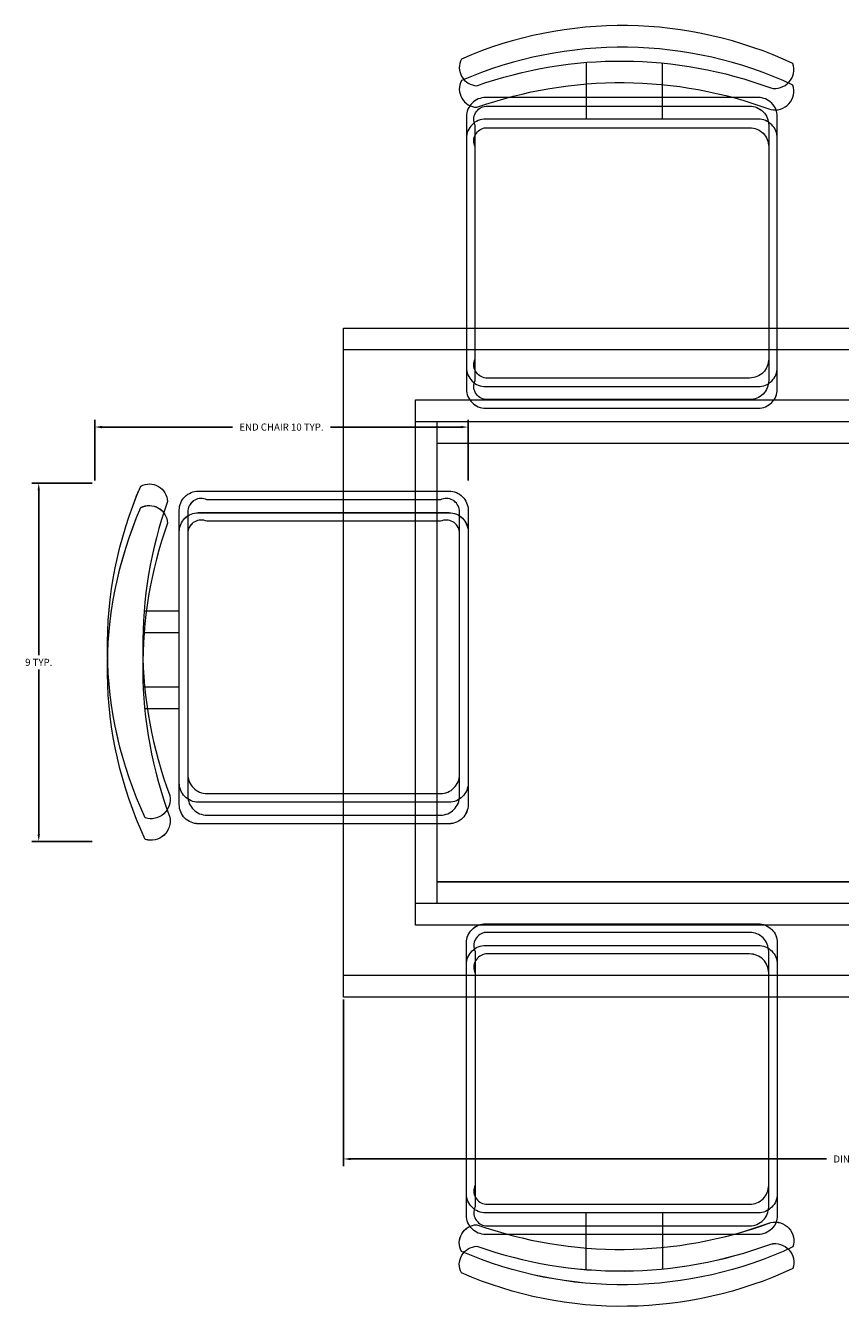
# Model space of a CAD drawing. Units: inches. Extents: x 2168 to 3056, y 1130 to 2629.
# Tile 13 of 42: x 2737 to 2758, y 1971 to 2003. Entities that reach past the tile are written whole.
import ezdxf

# ---------------------------------------------------------------- set-up
doc = ezdxf.new("R2010")
doc.units = ezdxf.units.IN
doc.layers.add('A-ANNO-DIMS', color=2, linetype='Continuous', lineweight=18)
doc.layers.add('A-FURN', color=8, linetype='Continuous', lineweight=13)
doc.styles.get("Standard").update_dxf_attribs({"font": 'arial.ttf'})
doc.dimstyles.get("Standard").update_dxf_attribs({"dimtxt": 0.18, "dimasz": 0.18, "dimexe": 0.18, "dimexo": 0.0625, "dimgap": 0.09, "dimtad": 0, "dimtih": 1, "dimtoh": 1, "dimdec": 4, "dimzin": 0, "dimdsep": 46, "dimtxsty": 'Standard', "dimcen": 0.09, "dimadec": 0, "dimazin": 0, "dimtfac": 1, "dimtdec": 4, "dimtofl": 0, "dimtmove": 0, "dimatfit": 3, "dimfxl": 1, "dimtolj": 1, "dimtzin": 0, "dimarcsym": 0})

# ---------------------------------------------------------------- blocks, each defined once
blk = doc.blocks.new('TABLE-DINING')
for points in [[(0, 17.016), (27.446, 17.016), (27.446, 0.549), (0, 0.549)], [(0, 17.016), (27.446, 17.016), (27.446, 0.549), (0, 0.549)], [(0, 16.467), (27.446, 16.467), (27.446, 0), (0, 0)], [(0, 16.467), (27.446, 16.467), (27.446, 0), (0, 0)], [(1.83, 15.187), (25.616, 15.187), (25.616, 2.379), (1.83, 2.379)], [(1.83, 15.186), (25.616, 15.186), (25.616, 2.378), (1.83, 2.378)], [(1.83, 14.638), (25.616, 14.638), (25.616, 1.83), (1.83, 1.83)], [(1.83, 14.637), (25.616, 14.637), (25.616, 1.829), (1.83, 1.829)], [(2.379, 14.638), (25.067, 14.638), (25.067, 2.928), (2.379, 2.928)], [(2.379, 14.637), (25.067, 14.637), (25.067, 2.927), (2.379, 2.927)], [(2.379, 14.089), (25.067, 14.089), (25.067, 2.379), (2.379, 2.379)], [(2.379, 14.089), (25.067, 14.089), (25.067, 2.378), (2.379, 2.378)]]:
    blk.add_lwpolyline(points, close=True)
blk = doc.blocks.new('CHAIR-DINING-END')
for points in [[(1.584, 1.138, -0.578392), (0.962, 0.571, -0.214524), (0.849, 9.01, -0.552014), (1.528, 8.613, 0.175809), (1.584, 1.138)], [(1.584, 1.138, -0.578392), (0.962, 0.571, -0.214524), (0.849, 9.009, -0.552014), (1.528, 8.613, 0.175809), (1.584, 1.138)], [(1.828, 8.395, -0.414214), (2.313, 8.88), (8.695, 8.88, -0.414214), (9.18, 8.395), (9.18, 1.455, -0.414214), (8.695, 0.969), (2.313, 0.969, -0.414214), (1.828, 1.455), (1.828, 8.395)], [(1.828, 8.395, -0.414214), (2.313, 8.88), (8.695, 8.88, -0.414214), (9.18, 8.395), (9.18, 1.455, -0.414214), (8.695, 0.969), (2.313, 0.969, -0.414214), (1.828, 1.455), (1.828, 8.395)], [(1.584, 0.589, -0.578392), (0.962, 0.023, -0.214524), (0.849, 8.461, -0.552014), (1.528, 8.064, 0.175809), (1.584, 0.589)], [(1.584, 0.589, -0.578392), (0.962, 0.022, -0.214524), (0.849, 8.46, -0.552014), (1.528, 8.064, 0.175809), (1.584, 0.589)], [(1.828, 7.846, -0.414214), (2.313, 8.332), (8.695, 8.332, -0.414214), (9.18, 7.846), (9.18, 0.906, -0.414214), (8.695, 0.421), (2.313, 0.421, -0.414214), (1.828, 0.906), (1.828, 7.846)], [(1.828, 7.846, -0.414214), (2.313, 8.331), (8.695, 8.331, -0.414214), (9.18, 7.846), (9.18, 0.906, -0.414214), (8.695, 0.42), (2.313, 0.42, -0.414214), (1.828, 0.906), (1.828, 7.846)], [(1.828, 3.893), (0.95, 3.893, 0.064759)], [(1.828, 3.892), (0.95, 3.892, 0.064759)], [(1.828, 3.344), (0.95, 3.344, 0.064759)], [(1.828, 3.343), (0.95, 3.343, 0.064759)]]:
    blk.add_lwpolyline(points, format="xyb")
for points in [[(2.047, 8.392), (2.047, 1.674, 0.414214), (2.532, 1.188), (8.476, 1.188, 0.414214), (8.961, 1.674), (8.961, 8.392, 0.512069), (8.476, 8.662), (2.532, 8.662, 0.512069)], [(2.047, 8.392), (2.047, 1.673, 0.414214), (2.532, 1.188), (8.476, 1.188, 0.414214), (8.961, 1.673), (8.961, 8.392, 0.512069), (8.476, 8.661), (2.532, 8.661, 0.512069)], [(2.047, 7.843), (2.047, 1.125, 0.414214), (2.532, 0.639), (8.476, 0.639, 0.414214), (8.961, 1.125), (8.961, 7.843, 0.512069), (8.476, 8.113), (2.532, 8.113, 0.512069)], [(2.047, 7.843), (2.047, 1.124, 0.414214), (2.532, 0.639), (8.476, 0.639, 0.414214), (8.961, 1.124), (8.961, 7.843, 0.512069), (8.476, 8.112), (2.532, 8.112, 0.512069)]]:
    blk.add_lwpolyline(points, format="xyb", close=True)
for points in [[(0.934, 5.835), (1.828, 5.835)], [(0.934, 5.835), (1.828, 5.835)], [(0.934, 5.286), (1.828, 5.286)], [(0.934, 5.286), (1.828, 5.286)]]:
    blk.add_lwpolyline(points)
blk = doc.blocks.new('*D24')
at = {"layer": 'A-ANNO-DIMS', "color": 0, "lineweight": -2, "transparency": 16777216}
for p, q in [((2744.965, 1978.514), (2744.965, 1974.279)), ((2772.411, 1978.514), (2772.411, 1974.279)), ((2745.145, 1974.459), (2757.257, 1974.459)), ((2772.231, 1974.459), (2760.12, 1974.459))]:
    blk.add_line(p, q, dxfattribs=at)
at = {"layer": 'A-ANNO-DIMS', "color": 0, "transparency": 16777216}
for points in [[(2745.145, 1974.489), (2745.145, 1974.429), (2744.965, 1974.459)], [(2772.231, 1974.489), (2772.231, 1974.429), (2772.411, 1974.459)]]:
    blk.add_solid(points, dxfattribs=at)
at = {"layer": 'Defpoints', "color": 0, "transparency": 16777216}
for p in [(2744.965, 1978.576), (2772.411, 1978.576), (2772.411, 1974.459)]:
    blk.add_point(p, dxfattribs=at)
at = {"layer": 'A-ANNO-DIMS', "color": 0, "transparency": 16777216, "insert": (2758.688, 1974.459), "char_height": 0.18, "attachment_point": 5}
blk.add_mtext('\\A1;DINING TABLE 27 TYP.', dxfattribs=at)
blk = doc.blocks.new('*D28')
at = {"layer": 'A-ANNO-DIMS', "color": 0, "lineweight": -2, "transparency": 16777216}
for p, q in [((2738.633, 1991.71), (2738.633, 1993.253)), ((2748.135, 1991.71), (2748.135, 1993.253)), ((2738.813, 1993.073), (2742.134, 1993.073)), ((2747.955, 1993.073), (2744.634, 1993.073))]:
    blk.add_line(p, q, dxfattribs=at)
at = {"layer": 'A-ANNO-DIMS', "color": 0, "transparency": 16777216}
for points in [[(2738.813, 1993.103), (2738.813, 1993.043), (2738.633, 1993.073)], [(2747.955, 1993.103), (2747.955, 1993.043), (2748.135, 1993.073)]]:
    blk.add_solid(points, dxfattribs=at)
at = {"layer": 'Defpoints', "color": 0, "transparency": 16777216}
for p in [(2748.135, 1993.073), (2738.633, 1991.647), (2748.135, 1991.647)]:
    blk.add_point(p, dxfattribs=at)
at = {"layer": 'A-ANNO-DIMS', "color": 0, "transparency": 16777216, "insert": (2743.384, 1993.073), "char_height": 0.18, "attachment_point": 5}
blk.add_mtext('\\A1;END CHAIR 10 TYP.', dxfattribs=at)
blk = doc.blocks.new('*D29')
at = {"layer": 'A-ANNO-DIMS', "color": 0, "lineweight": -2, "transparency": 16777216}
for p, q in [((2738.57, 1991.647), (2737.027, 1991.647)), ((2737.207, 1991.467), (2737.207, 1987.272)), ((2737.207, 1982.713), (2737.207, 1986.908)), ((2738.57, 1982.533), (2737.027, 1982.533))]:
    blk.add_line(p, q, dxfattribs=at)
at = {"layer": 'A-ANNO-DIMS', "color": 0, "transparency": 16777216}
for points in [[(2737.177, 1991.467), (2737.237, 1991.467), (2737.207, 1991.647)], [(2737.177, 1982.713), (2737.237, 1982.713), (2737.207, 1982.533)]]:
    blk.add_solid(points, dxfattribs=at)
at = {"layer": 'Defpoints', "color": 0, "transparency": 16777216}
for p in [(2737.207, 1991.647), (2738.633, 1991.647), (2738.633, 1982.533)]:
    blk.add_point(p, dxfattribs=at)
at = {"layer": 'A-ANNO-DIMS', "color": 0, "transparency": 16777216, "insert": (2737.207, 1987.09), "char_height": 0.18, "attachment_point": 5}
blk.add_mtext('\\A1;9 TYP.', dxfattribs=at)

msp = doc.modelspace()

# ---------------------------------------------------------------- linework, layer by layer
at = {"layer": 'A-FURN'}
for points in [[(2748.36, 2001.754, -0.175809), (2755.836, 2001.697, 0.578392), (2756.402, 2002.32, 0.214524), (2747.964, 2002.433, 0.552014), (2748.36, 2001.754, -0.065079)], [(2748.36, 2001.754, -0.175809), (2755.836, 2001.697, 0.578392), (2756.402, 2002.32, 0.214524), (2747.964, 2002.433, 0.552014), (2748.36, 2001.754, -0.065079)], [(2748.36, 2001.205, -0.175809), (2755.836, 2001.148, 0.578392), (2756.402, 2001.771, 0.214524), (2747.964, 2001.884, 0.552014), (2748.36, 2001.205, -0.065079)], [(2748.36, 2001.205, -0.175809), (2755.836, 2001.148, 0.578392), (2756.402, 2001.771, 0.214524), (2747.964, 2001.884, 0.552014), (2748.36, 2001.205, -0.065079)], [(2753.081, 2001.454), (2753.081, 2002.332, -0.064759)], [(2753.081, 2001.454), (2753.081, 2002.331, -0.064759)], [(2753.081, 2000.905), (2753.081, 2001.783, -0.064759)], [(2753.081, 2000.905), (2753.081, 2001.782, -0.064759)], [(2755.519, 2001.454), (2748.579, 2001.454, 0.414214), (2748.093, 2000.968), (2748.093, 1994.587, 0.414214), (2748.579, 1994.102), (2755.519, 1994.102, 0.414214), (2756.004, 1994.587), (2756.004, 2000.968, 0.414214), (2755.519, 2001.454)], [(2755.519, 2001.454), (2748.579, 2001.454, 0.414214), (2748.093, 2000.968), (2748.093, 1994.587, 0.414214), (2748.579, 1994.101), (2755.519, 1994.101, 0.414214), (2756.004, 1994.587), (2756.004, 2000.968, 0.414214), (2755.519, 2001.454)], [(2755.519, 2000.905), (2748.579, 2000.905, 0.414214), (2748.093, 2000.419), (2748.093, 1994.038, 0.414214), (2748.579, 1993.553), (2755.519, 1993.553, 0.414214), (2756.004, 1994.038), (2756.004, 2000.419, 0.414214), (2755.519, 2000.905)], [(2755.519, 2000.905), (2748.579, 2000.905, 0.414214), (2748.093, 2000.419), (2748.093, 1994.038, 0.414214), (2748.579, 1993.552), (2755.519, 1993.552, 0.414214), (2756.004, 1994.038), (2756.004, 2000.419, 0.414214), (2755.519, 2000.905)], [(2755.519, 1973.088), (2748.579, 1973.088, -0.414214), (2748.093, 1973.574), (2748.093, 1979.955, -0.414214), (2748.579, 1980.44), (2755.519, 1980.44, -0.414214), (2756.004, 1979.955), (2756.004, 1973.574, -0.414214), (2755.519, 1973.088)], [(2755.519, 1973.088), (2748.579, 1973.088, -0.414214), (2748.093, 1973.573), (2748.093, 1979.954, -0.414214), (2748.579, 1980.44), (2755.519, 1980.44, -0.414214), (2756.004, 1979.954), (2756.004, 1973.573, -0.414214), (2755.519, 1973.088)], [(2755.519, 1972.539), (2748.579, 1972.539, -0.414214), (2748.093, 1973.025), (2748.093, 1979.406, -0.414214), (2748.579, 1979.891), (2755.519, 1979.891, -0.414214), (2756.004, 1979.406), (2756.004, 1973.025, -0.414214), (2755.519, 1972.539)], [(2755.519, 1972.539), (2748.579, 1972.539, -0.414214), (2748.093, 1973.024), (2748.093, 1979.406, -0.414214), (2748.579, 1979.891), (2755.519, 1979.891, -0.414214), (2756.004, 1979.406), (2756.004, 1973.024, -0.414214), (2755.519, 1972.539)], [(2753.081, 1973.088), (2753.081, 1972.21, 0.064759)], [(2753.081, 1973.088), (2753.081, 1972.21, 0.064759)], [(2755.836, 1972.845, -0.578392), (2756.402, 1972.222, -0.214524), (2747.964, 1972.109, -0.552014), (2748.36, 1972.788, 0.175809), (2755.836, 1972.845)], [(2755.836, 1972.844, -0.578392), (2756.402, 1972.222, -0.214524), (2747.964, 1972.108, -0.552014), (2748.36, 1972.788, 0.175809), (2755.836, 1972.844)], [(2755.836, 1972.296, -0.578392), (2756.402, 1971.673, -0.214524), (2747.964, 1971.56, -0.552014), (2748.36, 1972.239, 0.175809), (2755.836, 1972.296)], [(2755.836, 1972.295, -0.578392), (2756.402, 1971.673, -0.214524), (2747.964, 1971.56, -0.552014), (2748.36, 1972.239, 0.175809), (2755.836, 1972.295)], [(2753.081, 1972.539), (2753.081, 1971.661, 0.064759)], [(2753.081, 1972.539), (2753.081, 1971.661, 0.064759)]]:
    msp.add_lwpolyline(points, format="xyb", dxfattribs=at)
for points in [[(2751.138, 2002.347), (2751.138, 2001.454)], [(2751.138, 2002.347), (2751.138, 2001.454)], [(2751.138, 2001.799), (2751.138, 2000.905)], [(2751.138, 2001.798), (2751.138, 2000.905)], [(2751.138, 1972.194), (2751.138, 1973.088)], [(2751.138, 1972.194), (2751.138, 1973.088)], [(2751.138, 1971.646), (2751.138, 1972.539)], [(2751.138, 1971.645), (2751.138, 1972.539)]]:
    msp.add_lwpolyline(points, dxfattribs=at)
for points in [[(2748.582, 2001.235), (2755.3, 2001.235, -0.414214), (2755.785, 2000.75), (2755.785, 1994.806, -0.414214), (2755.3, 1994.32), (2748.582, 1994.32, -0.512069), (2748.312, 1994.806), (2748.312, 2000.75, -0.512069)], [(2748.582, 2001.235), (2755.3, 2001.235, -0.414214), (2755.785, 2000.749), (2755.785, 1994.806, -0.414214), (2755.3, 1994.32), (2748.582, 1994.32, -0.512069), (2748.312, 1994.806), (2748.312, 2000.749, -0.512069)], [(2748.582, 2000.686), (2755.3, 2000.686, -0.414214), (2755.785, 2000.201), (2755.785, 1994.257, -0.414214), (2755.3, 1993.771), (2748.582, 1993.771, -0.512069), (2748.312, 1994.257), (2748.312, 2000.201, -0.512069)], [(2748.582, 2000.686), (2755.3, 2000.686, -0.414214), (2755.785, 2000.2), (2755.785, 1994.257, -0.414214), (2755.3, 1993.771), (2748.582, 1993.771, -0.512069), (2748.312, 1994.257), (2748.312, 2000.2, -0.512069)], [(2748.582, 1973.307), (2755.3, 1973.307, 0.414214), (2755.785, 1973.792), (2755.785, 1979.736, 0.414214), (2755.3, 1980.222), (2748.582, 1980.222, 0.512069), (2748.312, 1979.736), (2748.312, 1973.792, 0.512069)], [(2748.582, 1973.307), (2755.3, 1973.307, 0.414214), (2755.785, 1973.792), (2755.785, 1979.736, 0.414214), (2755.3, 1980.221), (2748.582, 1980.221, 0.512069), (2748.312, 1979.736), (2748.312, 1973.792, 0.512069)], [(2748.582, 1972.758), (2755.3, 1972.758, 0.414214), (2755.785, 1973.243), (2755.785, 1979.187, 0.414214), (2755.3, 1979.673), (2748.582, 1979.673, 0.512069), (2748.312, 1979.187), (2748.312, 1973.243, 0.512069)], [(2748.582, 1972.758), (2755.3, 1972.758, 0.414214), (2755.785, 1973.243), (2755.785, 1979.187, 0.414214), (2755.3, 1979.672), (2748.582, 1979.672, 0.512069), (2748.312, 1979.187), (2748.312, 1973.243, 0.512069)]]:
    msp.add_lwpolyline(points, format="xyb", close=True, dxfattribs=at)

# ---------------------------------------------------------------- block references
for name, p in [('TABLE-DINING', (2744.965, 1978.576)), ('CHAIR-DINING-END', (2738.955, 1982.564))]:
    msp.add_blockref(name, p, dxfattribs=at)

# ---------------------------------------------------------------- dimensions: what is measured, and where the dimension line sits
at = {"layer": 'A-ANNO-DIMS'}
for base, p1, p2, text, picture, middle in [((2748.135, 1993.073), (2738.633, 1991.647), (2748.135, 1991.647), 'END CHAIR <> TYP.', '*D28', (2743.384, 1993.073)), ((2772.411, 1974.459), (2744.965, 1978.576), (2772.411, 1978.576), 'DINING TABLE <> TYP.', '*D24', (2758.688, 1974.459))]:
    dim = msp.add_linear_dim(base=base, p1=p1, p2=p2, text=text, dimstyle='Standard', override={"dimdec": 0, "dimlfac": 1, "dimrnd": 0, "dimzin": 0, "dimdsep": 46, "dimlunit": 2}, dxfattribs=at)
    dim.commit()
    dim.dimension.update_dxf_attribs({"geometry": picture, "text_midpoint": middle})
dim = msp.add_linear_dim(base=(2737.207, 1991.647), p1=(2738.633, 1982.533), p2=(2738.633, 1991.647), angle=90, text='<> TYP.', dimstyle='Standard', override={"dimdec": 0, "dimlfac": 1, "dimrnd": 0, "dimzin": 0, "dimdsep": 46, "dimlunit": 2}, dxfattribs=at)
dim.commit()
dim.dimension.update_dxf_attribs({"geometry": '*D29', "text_midpoint": (2737.207, 1987.09)})

doc.saveas('drawing.dxf')
